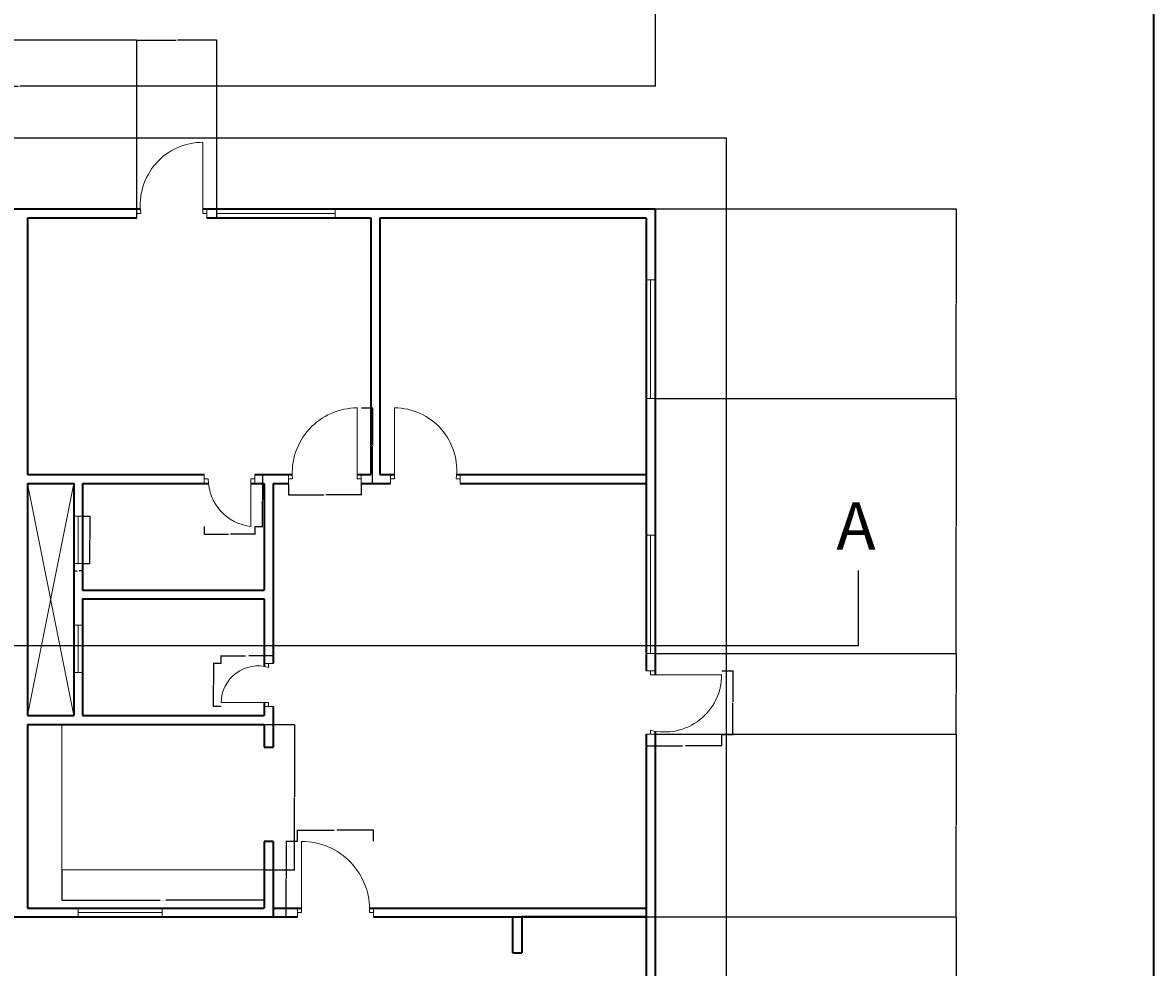
# Model space of a CAD drawing. Units: inches. Extents: x 1520 to 3401, y 1570 to 3432.
# Tile 14 of 15: x 2828 to 3401, y 2313 to 2791. Entities that reach past the tile are written whole.
import ezdxf

# ---------------------------------------------------------------- set-up
doc = ezdxf.new("R2010")
doc.units = ezdxf.units.IN
for name, color, linetype, lineweight in [('A-ANNO-DIMS', 2, 'Continuous', 18), ('A-ANNO-SYMB', 2, 'Continuous', 25), ('A-ANNO-TTLB', 7, 'Continuous', 35), ('A-DOOR', 3, 'Continuous', 18), ('A-FLOR-CASE', 8, 'Continuous', 18), ('A-FLOR-EDGE', 7, 'Continuous', 25), ('A-FLOR-EVTR', 7, 'Continuous', 35), ('A-FLOR-OPEN', 8, 'Continuous', 13), ('A-GLAZ', 4, 'Continuous', 18), ('A-WALL', 7, 'Continuous', 35)]:
    doc.layers.add(name, color=color, linetype=linetype, lineweight=lineweight)
doc.styles.get("Standard").update_dxf_attribs({"font": 'arial.ttf'})
doc.dimstyles.get("Standard").update_dxf_attribs({"dimtxt": 0.18, "dimasz": 0.18, "dimexe": 0.18, "dimexo": 0.0625, "dimgap": 0.09, "dimtad": 0, "dimtih": 1, "dimtoh": 1, "dimdec": 4, "dimzin": 0, "dimdsep": 46, "dimtxsty": 'Standard', "dimcen": 0.09, "dimadec": 0, "dimazin": 0, "dimtfac": 1, "dimtdec": 4, "dimtofl": 0, "dimtmove": 0, "dimatfit": 3, "dimfxl": 1, "dimtolj": 1, "dimtzin": 0, "dimarcsym": 0})

# ---------------------------------------------------------------- blocks, each defined once
blk = doc.blocks.new('DOOR-SWING-36-05')
for p, q in [((34.83, 2.25), (34.83, 38.25)), ((0, 4.5), (0, 4.5)), ((0, 4.5), (0, 0)), ((0, 0), (0, 2.25)), ((0, 2.25), (2, 2.25)), ((36.83, 2.25), (34.83, 2.25)), ((36.83, 4.5), (36.83, 0)), ((36.83, 0), (36.83, 2.25))]:
    blk.add_line(p, q)
blk.add_arc((34.83, 5.28), 32.97, 90, 185.2728)
blk = doc.blocks.new('DOOR-SWING-36-06')
for p, q in [((2, 2.25), (2, 38.25)), ((0, 4.5), (0, 0)), ((0, 0), (0, 2.25)), ((0, 2.25), (2, 2.25)), ((35.31, 2.25), (33.31, 2.25)), ((35.31, 4.5), (35.31, 0)), ((35.31, 0), (35.31, 2.25))]:
    blk.add_line(p, q)
blk.add_arc((2, 6.63), 31.62, 352.0372, 90)
blk = doc.blocks.new('DOOR-SWING-24-07')
for p, q in [((21.75, 21.72), (26.25, 21.72)), ((26.25, 21.72), (24, 21.72)), ((24, 21.72), (24, 19.72)), ((24, 2), (0, 2)), ((21.75, 0), (26.25, 0)), ((24, 0), (24, 2)), ((26.25, 0), (24, 0))]:
    blk.add_line(p, q)
blk.add_arc((18.54, 2), 18.54, 72.8832, 180)
blk = doc.blocks.new('DOOR-SWING-24-08')
for p, q in [((0, 26.25), (0, 21.75)), ((0, 21.75), (0, 24)), ((0, 24), (2, 24)), ((25.6, 24), (23.6, 24)), ((23.6, 24), (23.6, 0)), ((25.6, 21.75), (25.6, 26.25)), ((25.6, 26.25), (25.6, 24))]:
    blk.add_line(p, q)
blk.add_arc((26.13, 24), 24.13, 180, 263.9827)
blk = doc.blocks.new('DOOR-SWING-36-20')
for p, q in [((2, 2.25), (2, 38.25)), ((0, 4.5), (0, 0)), ((0, 0), (0, 2.25)), ((0, 2.25), (2, 2.25)), ((38.43, 2.25), (36.43, 2.25)), ((38.43, 4.5), (38.43, 0)), ((38.43, 0), (38.43, 2.25))]:
    blk.add_line(p, q)
blk.add_arc((2, 3.79), 34.46, 357.4431, 90)
blk = doc.blocks.new('DOOR-SWING-36-21')
for p, q in [((33.5, 2.25), (33.5, 38.25)), ((0, 4.5), (0, 0)), ((0, 0), (0, 2.25)), ((0, 2.25), (2, 2.25)), ((35.5, 2.25), (33.5, 2.25)), ((35.5, 0), (35.5, 4.5)), ((35.5, 4.5), (35.5, 2.25))]:
    blk.add_line(p, q)
blk.add_arc((33.5, 6.47), 31.78, 90, 187.6316)
blk = doc.blocks.new('DOOR-SWING-36-23')
for p, q in [((0, 32.12), (4.5, 32.12)), ((4.5, 32.12), (2.25, 32.12)), ((2.25, 32.12), (2.25, 30.12)), ((2.25, 30.12), (38.25, 30.12)), ((4.5, 0), (0, 0)), ((0, 0), (2.25, 0)), ((2.25, 0), (2.25, 2))]:
    blk.add_line(p, q)
blk.add_arc((9.27, 30.12), 28.98, 255.986, 0)
blk = doc.blocks.new('WIN-PLAN-24-01')
for p, q in [((0, 4.5), (0, 0)), ((0, 0), (0, 2.25)), ((0, 2.25), (24, 2.25)), ((24, 2.25), (24, 4.5)), ((24, 4.5), (24, 0))]:
    blk.add_line(p, q)
blk = doc.blocks.new('WIN-PLAN-60-02')
for p, q in [((4.5, 60), (0, 60)), ((0, 60), (2.25, 60)), ((2.25, 60), (2.25, 0)), ((4.5, 0), (0, 0)), ((2.25, 0), (4.5, 0))]:
    blk.add_line(p, q)
blk = doc.blocks.new('WIN-PLAN-60-03')
for p, q in [((0, 2.25), (0, 4.5)), ((0, 4.5), (0, 0)), ((60, 2.25), (0, 2.25)), ((60, 0), (60, 4.5)), ((60, 4.5), (60, 2.25))]:
    blk.add_line(p, q)
blk = doc.blocks.new('WIN-PLAN-24-07')
for p, q in [((2.25, 24), (0, 24)), ((0, 24), (4.5, 24)), ((2.25, 0), (2.25, 24)), ((4.5, 0), (0, 0)), ((0, 0), (4.5, 0)), ((4.5, 0), (2.25, 0))]:
    blk.add_line(p, q)
blk = doc.blocks.new('WIN-PLAN-42.5-08')
for p, q in [((0, 4.5), (0, 0)), ((0, 0), (0, 2.25)), ((0, 2.25), (0, 2.25)), ((0, 2.25), (42.53, 2.25)), ((42.53, 0), (42.53, 4.5))]:
    blk.add_line(p, q)
blk = doc.blocks.new('KITCHEN-COUNTER-03')
for p, q in [((0, 0), (0, 73.56)), ((102.45, 0), (0, 0))]:
    blk.add_line(p, q)
blk = doc.blocks.new('*D89')
at = {"layer": 'A-ANNO-DIMS', "color": 0, "lineweight": -2, "transparency": 16777216}
for p, q in [((2999.61, 2596.43), (3005.47, 2596.43)), ((3005.29, 2596.25), (3005.29, 2577.49)), ((3005.29, 2558.36), (3005.29, 2577.12)), ((2999.61, 2558.18), (3005.47, 2558.18))]:
    blk.add_line(p, q, dxfattribs=at)
at = {"layer": 'A-ANNO-DIMS', "color": 0, "transparency": 16777216}
for points in [[(3005.26, 2596.25), (3005.32, 2596.25), (3005.29, 2596.43)], [(3005.26, 2558.36), (3005.32, 2558.36), (3005.29, 2558.18)]]:
    blk.add_solid(points, dxfattribs=at)
at = {"layer": 'Defpoints', "color": 0, "transparency": 16777216}
for p in [(2999.55, 2596.43), (3005.29, 2596.43), (2999.55, 2558.18)]:
    blk.add_point(p, dxfattribs=at)
at = {"layer": 'A-ANNO-DIMS', "color": 0, "transparency": 16777216, "insert": (3005.29, 2577.3), "char_height": 0.18, "attachment_point": 5}
blk.add_mtext('\\A1;D05 38 TYP.', dxfattribs=at)
blk = doc.blocks.new('*D90')
at = {"layer": 'A-ANNO-DIMS', "color": 0, "lineweight": -2, "transparency": 16777216}
for p, q in [((2962.72, 2558.12), (2962.72, 2552.26)), ((2999.55, 2558.12), (2999.55, 2552.26)), ((2962.9, 2552.44), (2980.61, 2552.44)), ((2999.37, 2552.44), (2981.66, 2552.44))]:
    blk.add_line(p, q, dxfattribs=at)
at = {"layer": 'A-ANNO-DIMS', "color": 0, "transparency": 16777216}
for points in [[(2962.9, 2552.47), (2962.9, 2552.41), (2962.72, 2552.44)], [(2999.37, 2552.47), (2999.37, 2552.41), (2999.55, 2552.44)]]:
    blk.add_solid(points, dxfattribs=at)
at = {"layer": 'Defpoints', "color": 0, "transparency": 16777216}
for p in [(2962.72, 2558.18), (2999.55, 2558.18), (2999.55, 2552.44)]:
    blk.add_point(p, dxfattribs=at)
at = {"layer": 'A-ANNO-DIMS', "color": 0, "transparency": 16777216, "insert": (2981.14, 2552.44), "char_height": 0.18, "attachment_point": 5}
blk.add_mtext('\\A1;37 TYP.', dxfattribs=at)
blk = doc.blocks.new('*D93')
at = {"layer": 'A-ANNO-DIMS', "color": 0, "lineweight": -2, "transparency": 16777216}
for p, q in [((2928.65, 2467.04), (2928.65, 2471.1)), ((2928.83, 2470.92), (2940.98, 2470.92)), ((2954.72, 2470.92), (2942.56, 2470.92)), ((2954.9, 2467.04), (2954.9, 2471.1))]:
    blk.add_line(p, q, dxfattribs=at)
at = {"layer": 'A-ANNO-DIMS', "color": 0, "transparency": 16777216}
for points in [[(2928.83, 2470.95), (2928.83, 2470.89), (2928.65, 2470.92)], [(2954.72, 2470.95), (2954.72, 2470.89), (2954.9, 2470.92)]]:
    blk.add_solid(points, dxfattribs=at)
at = {"layer": 'Defpoints', "color": 0, "transparency": 16777216}
for p in [(2954.9, 2470.92), (2928.65, 2466.98), (2954.9, 2466.98)]:
    blk.add_point(p, dxfattribs=at)
at = {"layer": 'A-ANNO-DIMS', "color": 0, "transparency": 16777216, "insert": (2941.77, 2470.92), "char_height": 0.18, "attachment_point": 5}
blk.add_mtext('\\A1;D07 26 TYP.', dxfattribs=at)
blk = doc.blocks.new('*D94')
at = {"layer": 'A-ANNO-DIMS', "color": 0, "lineweight": -2, "transparency": 16777216}
for p, q in [((2928.59, 2466.98), (2924.53, 2466.98)), ((2924.71, 2466.8), (2924.71, 2456.3)), ((2924.71, 2445.44), (2924.71, 2455.94)), ((2928.59, 2445.26), (2924.53, 2445.26))]:
    blk.add_line(p, q, dxfattribs=at)
at = {"layer": 'A-ANNO-DIMS', "color": 0, "transparency": 16777216}
for points in [[(2924.68, 2466.8), (2924.74, 2466.8), (2924.71, 2466.98)], [(2924.68, 2445.44), (2924.74, 2445.44), (2924.71, 2445.26)]]:
    blk.add_solid(points, dxfattribs=at)
at = {"layer": 'Defpoints', "color": 0, "transparency": 16777216}
for p in [(2924.71, 2466.98), (2928.65, 2466.98), (2928.65, 2445.26)]:
    blk.add_point(p, dxfattribs=at)
at = {"layer": 'A-ANNO-DIMS', "color": 0, "transparency": 16777216, "insert": (2924.71, 2456.12), "char_height": 0.18, "attachment_point": 5}
blk.add_mtext('\\A1;22 TYP.', dxfattribs=at)
blk = doc.blocks.new('*D95')
at = {"layer": 'A-ANNO-DIMS', "color": 0, "lineweight": -2, "transparency": 16777216}
for p, q in [((2945.71, 2562.68), (2949.77, 2562.68)), ((2949.59, 2562.5), (2949.59, 2549.74)), ((2949.59, 2536.61), (2949.59, 2549.37)), ((2945.71, 2536.43), (2949.77, 2536.43))]:
    blk.add_line(p, q, dxfattribs=at)
at = {"layer": 'A-ANNO-DIMS', "color": 0, "transparency": 16777216}
for points in [[(2949.56, 2562.5), (2949.62, 2562.5), (2949.59, 2562.68)], [(2949.56, 2536.61), (2949.62, 2536.61), (2949.59, 2536.43)]]:
    blk.add_solid(points, dxfattribs=at)
at = {"layer": 'Defpoints', "color": 0, "transparency": 16777216}
for p in [(2945.65, 2562.68), (2949.59, 2562.68), (2945.65, 2536.43)]:
    blk.add_point(p, dxfattribs=at)
at = {"layer": 'A-ANNO-DIMS', "color": 0, "transparency": 16777216, "insert": (2949.59, 2549.55), "char_height": 0.18, "attachment_point": 5}
blk.add_mtext('\\A1;D08 26 TYP.', dxfattribs=at)
blk = doc.blocks.new('*D96')
at = {"layer": 'A-ANNO-DIMS', "color": 0, "lineweight": -2, "transparency": 16777216}
for p, q in [((2920.05, 2536.37), (2920.05, 2532.31)), ((2920.23, 2532.49), (2932.32, 2532.49)), ((2945.47, 2532.49), (2933.38, 2532.49)), ((2945.65, 2536.37), (2945.65, 2532.31))]:
    blk.add_line(p, q, dxfattribs=at)
at = {"layer": 'A-ANNO-DIMS', "color": 0, "transparency": 16777216}
for points in [[(2920.23, 2532.52), (2920.23, 2532.46), (2920.05, 2532.49)], [(2945.47, 2532.52), (2945.47, 2532.46), (2945.65, 2532.49)]]:
    blk.add_solid(points, dxfattribs=at)
at = {"layer": 'Defpoints', "color": 0, "transparency": 16777216}
for p in [(2920.05, 2536.43), (2945.65, 2536.43), (2945.65, 2532.49)]:
    blk.add_point(p, dxfattribs=at)
at = {"layer": 'A-ANNO-DIMS', "color": 0, "transparency": 16777216, "insert": (2932.85, 2532.49), "char_height": 0.18, "attachment_point": 5}
blk.add_mtext('\\A1;26 TYP.', dxfattribs=at)
blk = doc.blocks.new('*D119')
at = {"layer": 'A-ANNO-DIMS', "color": 0, "lineweight": -2, "transparency": 16777216}
for p, q in [((2967.34, 2376.99), (2967.34, 2382.87)), ((2967.52, 2382.69), (2985.76, 2382.69)), ((3005.59, 2382.69), (2987.34, 2382.69)), ((3005.77, 2376.99), (3005.77, 2382.87))]:
    blk.add_line(p, q, dxfattribs=at)
at = {"layer": 'A-ANNO-DIMS', "color": 0, "transparency": 16777216}
for points in [[(2967.52, 2382.72), (2967.52, 2382.66), (2967.34, 2382.69)], [(3005.59, 2382.72), (3005.59, 2382.66), (3005.77, 2382.69)]]:
    blk.add_solid(points, dxfattribs=at)
at = {"layer": 'Defpoints', "color": 0, "transparency": 16777216}
for p in [(3005.77, 2382.69), (2967.34, 2376.93), (3005.77, 2376.93)]:
    blk.add_point(p, dxfattribs=at)
at = {"layer": 'A-ANNO-DIMS', "color": 0, "transparency": 16777216, "insert": (2986.55, 2382.69), "char_height": 0.18, "attachment_point": 5}
blk.add_mtext('\\A1;D20 38 TYP.', dxfattribs=at)
blk = doc.blocks.new('*D120')
at = {"layer": 'A-ANNO-DIMS', "color": 0, "lineweight": -2, "transparency": 16777216}
for p, q in [((2967.28, 2376.93), (2961.39, 2376.93)), ((2961.57, 2376.75), (2961.57, 2357.99)), ((2961.57, 2338.86), (2961.57, 2357.62)), ((2967.28, 2338.68), (2961.39, 2338.68))]:
    blk.add_line(p, q, dxfattribs=at)
at = {"layer": 'A-ANNO-DIMS', "color": 0, "transparency": 16777216}
for points in [[(2961.54, 2376.75), (2961.6, 2376.75), (2961.57, 2376.93)], [(2961.54, 2338.86), (2961.6, 2338.86), (2961.57, 2338.68)]]:
    blk.add_solid(points, dxfattribs=at)
at = {"layer": 'Defpoints', "color": 0, "transparency": 16777216}
for p in [(2961.57, 2376.93), (2967.34, 2376.93), (2967.34, 2338.68)]:
    blk.add_point(p, dxfattribs=at)
at = {"layer": 'A-ANNO-DIMS', "color": 0, "transparency": 16777216, "insert": (2961.57, 2357.8), "char_height": 0.18, "attachment_point": 5}
blk.add_mtext('\\A1;38 TYP.', dxfattribs=at)
blk = doc.blocks.new('*D125')
at = {"layer": 'A-ANNO-DIMS', "color": 0, "lineweight": -2, "transparency": 16777216}
for p, q in [((3143.9, 2430.96), (3143.9, 2425.11)), ((3182.15, 2430.96), (3182.15, 2425.11)), ((3144.08, 2425.29), (3162.23, 2425.29)), ((3181.97, 2425.29), (3163.81, 2425.29))]:
    blk.add_line(p, q, dxfattribs=at)
at = {"layer": 'A-ANNO-DIMS', "color": 0, "transparency": 16777216}
for points in [[(3144.08, 2425.32), (3144.08, 2425.26), (3143.9, 2425.29)], [(3181.97, 2425.32), (3181.97, 2425.26), (3182.15, 2425.29)]]:
    blk.add_solid(points, dxfattribs=at)
at = {"layer": 'Defpoints', "color": 0, "transparency": 16777216}
for p in [(3143.9, 2431.03), (3182.15, 2431.03), (3182.15, 2425.29)]:
    blk.add_point(p, dxfattribs=at)
at = {"layer": 'A-ANNO-DIMS', "color": 0, "transparency": 16777216, "insert": (3163.02, 2425.29), "char_height": 0.18, "attachment_point": 5}
blk.add_mtext('\\A1;D23 38 TYP.', dxfattribs=at)
blk = doc.blocks.new('*D126')
at = {"layer": 'A-ANNO-DIMS', "color": 0, "lineweight": -2, "transparency": 16777216}
for p, q in [((3182.21, 2463.31), (3188.07, 2463.31)), ((3187.89, 2463.13), (3187.89, 2447.35)), ((3187.89, 2431.21), (3187.89, 2446.98)), ((3182.21, 2431.03), (3188.07, 2431.03))]:
    blk.add_line(p, q, dxfattribs=at)
at = {"layer": 'A-ANNO-DIMS', "color": 0, "transparency": 16777216}
for points in [[(3187.86, 2463.13), (3187.92, 2463.13), (3187.89, 2463.31)], [(3187.86, 2431.21), (3187.92, 2431.21), (3187.89, 2431.03)]]:
    blk.add_solid(points, dxfattribs=at)
at = {"layer": 'Defpoints', "color": 0, "transparency": 16777216}
for p in [(3182.15, 2463.31), (3187.89, 2463.31), (3182.15, 2431.03)]:
    blk.add_point(p, dxfattribs=at)
at = {"layer": 'A-ANNO-DIMS', "color": 0, "transparency": 16777216, "insert": (3187.89, 2447.17), "char_height": 0.18, "attachment_point": 5}
blk.add_mtext('\\A1;32 TYP.', dxfattribs=at)
blk = doc.blocks.new('*D145')
at = {"layer": 'A-ANNO-DIMS', "color": 0, "lineweight": -2, "transparency": 16777216}
for p, q in [((2858.46, 2541.57), (2862.18, 2541.57)), ((2862, 2541.39), (2862, 2529.75)), ((2862, 2517.75), (2862, 2529.39)), ((2858.46, 2517.57), (2862.18, 2517.57))]:
    blk.add_line(p, q, dxfattribs=at)
at = {"layer": 'A-ANNO-DIMS', "color": 0, "transparency": 16777216}
for points in [[(2861.97, 2541.39), (2862.03, 2541.39), (2862, 2541.57)], [(2861.97, 2517.75), (2862.03, 2517.75), (2862, 2517.57)]]:
    blk.add_solid(points, dxfattribs=at)
at = {"layer": 'Defpoints', "color": 0, "transparency": 16777216}
for p in [(2858.4, 2541.57), (2862, 2541.57), (2858.4, 2517.57)]:
    blk.add_point(p, dxfattribs=at)
at = {"layer": 'A-ANNO-DIMS', "color": 0, "transparency": 16777216, "insert": (2862, 2529.57), "char_height": 0.18, "attachment_point": 5}
blk.add_mtext('\\A1;W7 24 TYP.', dxfattribs=at)
blk = doc.blocks.new('*D146')
at = {"layer": 'A-ANNO-DIMS', "color": 0, "lineweight": -2, "transparency": 16777216}
for p, q in [((2853.9, 2517.5), (2853.9, 2513.79)), ((2858.4, 2517.5), (2858.4, 2513.79)), ((2854.08, 2513.97), (2855.69, 2513.97)), ((2858.22, 2513.97), (2856.61, 2513.97))]:
    blk.add_line(p, q, dxfattribs=at)
at = {"layer": 'A-ANNO-DIMS', "color": 0, "transparency": 16777216}
for points in [[(2854.08, 2514), (2854.08, 2513.94), (2853.9, 2513.97)], [(2858.22, 2514), (2858.22, 2513.94), (2858.4, 2513.97)]]:
    blk.add_solid(points, dxfattribs=at)
at = {"layer": 'Defpoints', "color": 0, "transparency": 16777216}
for p in [(2853.9, 2517.57), (2858.4, 2517.57), (2858.4, 2513.97)]:
    blk.add_point(p, dxfattribs=at)
at = {"layer": 'A-ANNO-DIMS', "color": 0, "transparency": 16777216, "insert": (2856.15, 2513.97), "char_height": 0.18, "attachment_point": 5}
blk.add_mtext('\\A1;5 TYP.', dxfattribs=at)
blk = doc.blocks.new('*D153')
at = {"layer": 'A-ANNO-DIMS', "color": 0, "lineweight": -2, "transparency": 16777216}
for p, q in [((2847.95, 2362.55), (2847.95, 2347.07)), ((2950.4, 2362.55), (2950.4, 2347.07)), ((2848.13, 2347.25), (2897.72, 2347.25)), ((2950.22, 2347.25), (2900.62, 2347.25))]:
    blk.add_line(p, q, dxfattribs=at)
at = {"layer": 'A-ANNO-DIMS', "color": 0, "transparency": 16777216}
for points in [[(2848.13, 2347.28), (2848.13, 2347.22), (2847.95, 2347.25)], [(2950.22, 2347.28), (2950.22, 2347.22), (2950.4, 2347.25)]]:
    blk.add_solid(points, dxfattribs=at)
at = {"layer": 'Defpoints', "color": 0, "transparency": 16777216}
for p in [(2847.95, 2362.61), (2950.4, 2362.61), (2950.4, 2347.25)]:
    blk.add_point(p, dxfattribs=at)
at = {"layer": 'A-ANNO-DIMS', "color": 0, "transparency": 16777216, "insert": (2899.17, 2347.25), "char_height": 0.18, "attachment_point": 5}
blk.add_mtext('\\A1;COUNTER C3 102 TYP.', dxfattribs=at)
blk = doc.blocks.new('*D154')
at = {"layer": 'A-ANNO-DIMS', "color": 0, "lineweight": -2, "transparency": 16777216}
for p, q in [((2950.46, 2436.18), (2965.95, 2436.18)), ((2965.77, 2436), (2965.77, 2399.58)), ((2965.77, 2362.79), (2965.77, 2399.22)), ((2950.46, 2362.61), (2965.95, 2362.61))]:
    blk.add_line(p, q, dxfattribs=at)
at = {"layer": 'A-ANNO-DIMS', "color": 0, "transparency": 16777216}
for points in [[(2965.74, 2436), (2965.8, 2436), (2965.77, 2436.18)], [(2965.74, 2362.79), (2965.8, 2362.79), (2965.77, 2362.61)]]:
    blk.add_solid(points, dxfattribs=at)
at = {"layer": 'Defpoints', "color": 0, "transparency": 16777216}
for p in [(2950.4, 2436.18), (2965.77, 2436.18), (2950.4, 2362.61)]:
    blk.add_point(p, dxfattribs=at)
at = {"layer": 'A-ANNO-DIMS', "color": 0, "transparency": 16777216, "insert": (2965.77, 2399.4), "char_height": 0.18, "attachment_point": 5}
blk.add_mtext('\\A1;74 TYP.', dxfattribs=at)
blk = doc.blocks.new('*D197')
at = {"layer": 'A-ANNO-DIMS', "color": 0, "lineweight": -2, "transparency": 16777216}
for p, q in [((3143.96, 2338.68), (3301.09, 2338.68)), ((3300.91, 2338.5), (3300.91, 2288.86)), ((3300.91, 2238.86), (3300.91, 2288.5)), ((3143.96, 2238.68), (3301.09, 2238.68))]:
    blk.add_line(p, q, dxfattribs=at)
at = {"layer": 'A-ANNO-DIMS', "color": 0, "transparency": 16777216}
for points in [[(3300.88, 2338.5), (3300.94, 2338.5), (3300.91, 2338.68)], [(3300.88, 2238.86), (3300.94, 2238.86), (3300.91, 2238.68)]]:
    blk.add_solid(points, dxfattribs=at)
at = {"layer": 'Defpoints', "color": 0, "transparency": 16777216}
for p in [(3143.9, 2338.68), (3300.91, 2338.68), (3143.9, 2238.68)]:
    blk.add_point(p, dxfattribs=at)
at = {"layer": 'A-ANNO-DIMS', "color": 0, "transparency": 16777216, "insert": (3300.91, 2288.68), "char_height": 0.18, "attachment_point": 5}
blk.add_mtext('\\A1;100', dxfattribs=at)
blk = doc.blocks.new('*D198')
at = {"layer": 'A-ANNO-DIMS', "color": 0, "lineweight": -2, "transparency": 16777216}
for p, q in [((3148.46, 2431.19), (3301.09, 2431.19)), ((3300.91, 2431.01), (3300.91, 2385.11)), ((3300.91, 2338.86), (3300.91, 2384.75)), ((3143.96, 2338.68), (3301.09, 2338.68))]:
    blk.add_line(p, q, dxfattribs=at)
at = {"layer": 'A-ANNO-DIMS', "color": 0, "transparency": 16777216}
for points in [[(3300.88, 2431.01), (3300.94, 2431.01), (3300.91, 2431.19)], [(3300.88, 2338.86), (3300.94, 2338.86), (3300.91, 2338.68)]]:
    blk.add_solid(points, dxfattribs=at)
at = {"layer": 'Defpoints', "color": 0, "transparency": 16777216}
for p in [(3148.4, 2431.19), (3300.91, 2431.19), (3143.9, 2338.68)]:
    blk.add_point(p, dxfattribs=at)
at = {"layer": 'A-ANNO-DIMS', "color": 0, "transparency": 16777216, "insert": (3300.91, 2384.93), "char_height": 0.18, "attachment_point": 5}
blk.add_mtext('\\A1;92.5', dxfattribs=at)
blk = doc.blocks.new('*D199')
at = {"layer": 'A-ANNO-DIMS', "color": 0, "lineweight": -2, "transparency": 16777216}
for p, q in [((3148.46, 2472.01), (3301.09, 2472.01)), ((3300.91, 2471.83), (3300.91, 2451.78)), ((3300.91, 2431.37), (3300.91, 2451.42)), ((3148.46, 2431.19), (3301.09, 2431.19))]:
    blk.add_line(p, q, dxfattribs=at)
at = {"layer": 'A-ANNO-DIMS', "color": 0, "transparency": 16777216}
for points in [[(3300.88, 2471.83), (3300.94, 2471.83), (3300.91, 2472.01)], [(3300.88, 2431.37), (3300.94, 2431.37), (3300.91, 2431.19)]]:
    blk.add_solid(points, dxfattribs=at)
at = {"layer": 'Defpoints', "color": 0, "transparency": 16777216}
for p in [(3148.4, 2472.01), (3300.91, 2472.01), (3148.4, 2431.19)]:
    blk.add_point(p, dxfattribs=at)
at = {"layer": 'A-ANNO-DIMS', "color": 0, "transparency": 16777216, "insert": (3300.91, 2451.6), "char_height": 0.18, "attachment_point": 5}
blk.add_mtext('\\A1;40.83', dxfattribs=at)
blk = doc.blocks.new('*D200')
at = {"layer": 'A-ANNO-DIMS', "color": 0, "lineweight": -2, "transparency": 16777216}
for p, q in [((3148.46, 2601.18), (3301.09, 2601.18)), ((3300.91, 2601), (3300.91, 2536.78)), ((3300.91, 2472.19), (3300.91, 2536.42)), ((3148.46, 2472.01), (3301.09, 2472.01))]:
    blk.add_line(p, q, dxfattribs=at)
at = {"layer": 'A-ANNO-DIMS', "color": 0, "transparency": 16777216}
for points in [[(3300.88, 2601), (3300.94, 2601), (3300.91, 2601.18)], [(3300.88, 2472.19), (3300.94, 2472.19), (3300.91, 2472.01)]]:
    blk.add_solid(points, dxfattribs=at)
at = {"layer": 'Defpoints', "color": 0, "transparency": 16777216}
for p in [(3148.4, 2601.18), (3300.91, 2601.18), (3148.4, 2472.01)]:
    blk.add_point(p, dxfattribs=at)
at = {"layer": 'A-ANNO-DIMS', "color": 0, "transparency": 16777216, "insert": (3300.91, 2536.6), "char_height": 0.18, "attachment_point": 5}
blk.add_mtext('\\A1;129.17', dxfattribs=at)
blk = doc.blocks.new('*D201')
at = {"layer": 'A-ANNO-DIMS', "color": 0, "lineweight": -2, "transparency": 16777216}
for p, q in [((3148.46, 2697.18), (3301.09, 2697.18)), ((3300.91, 2697), (3300.91, 2649.36)), ((3300.91, 2601.36), (3300.91, 2649)), ((3148.46, 2601.18), (3301.09, 2601.18))]:
    blk.add_line(p, q, dxfattribs=at)
at = {"layer": 'A-ANNO-DIMS', "color": 0, "transparency": 16777216}
for points in [[(3300.88, 2697), (3300.94, 2697), (3300.91, 2697.18)], [(3300.88, 2601.36), (3300.94, 2601.36), (3300.91, 2601.18)]]:
    blk.add_solid(points, dxfattribs=at)
at = {"layer": 'Defpoints', "color": 0, "transparency": 16777216}
for p in [(3148.4, 2697.18), (3300.91, 2697.18), (3148.4, 2601.18)]:
    blk.add_point(p, dxfattribs=at)
at = {"layer": 'A-ANNO-DIMS', "color": 0, "transparency": 16777216, "insert": (3300.91, 2649.18), "char_height": 0.18, "attachment_point": 5}
blk.add_mtext('\\A1;96', dxfattribs=at)
blk = doc.blocks.new('*D205')
at = {"layer": 'A-ANNO-DIMS', "color": 0, "lineweight": -2, "transparency": 16777216}
for p, q in [((2733.5, 2697.24), (2733.5, 2782.76)), ((2733.68, 2782.58), (2809.22, 2782.58)), ((2885.68, 2782.58), (2810.13, 2782.58)), ((2885.86, 2692.74), (2885.86, 2782.76))]:
    blk.add_line(p, q, dxfattribs=at)
at = {"layer": 'A-ANNO-DIMS', "color": 0, "transparency": 16777216}
for points in [[(2733.68, 2782.61), (2733.68, 2782.55), (2733.5, 2782.58)], [(2885.68, 2782.61), (2885.68, 2782.55), (2885.86, 2782.58)]]:
    blk.add_solid(points, dxfattribs=at)
at = {"layer": 'Defpoints', "color": 0, "transparency": 16777216}
for p in [(2885.86, 2782.58), (2733.5, 2697.18), (2885.86, 2692.68)]:
    blk.add_point(p, dxfattribs=at)
at = {"layer": 'A-ANNO-DIMS', "color": 0, "transparency": 16777216, "insert": (2809.68, 2782.58), "char_height": 0.18, "attachment_point": 5}
blk.add_mtext('\\A1;152.37', dxfattribs=at)
blk = doc.blocks.new('*D206')
at = {"layer": 'A-ANNO-DIMS', "color": 0, "lineweight": -2, "transparency": 16777216}
for p, q in [((2885.86, 2692.74), (2885.86, 2782.76)), ((2886.04, 2782.58), (2905.74, 2782.58)), ((2926.19, 2782.58), (2906.5, 2782.58)), ((2926.37, 2692.74), (2926.37, 2782.76))]:
    blk.add_line(p, q, dxfattribs=at)
at = {"layer": 'A-ANNO-DIMS', "color": 0, "transparency": 16777216}
for points in [[(2886.04, 2782.61), (2886.04, 2782.55), (2885.86, 2782.58)], [(2926.19, 2782.61), (2926.19, 2782.55), (2926.37, 2782.58)]]:
    blk.add_solid(points, dxfattribs=at)
at = {"layer": 'Defpoints', "color": 0, "transparency": 16777216}
for p in [(2926.37, 2782.58), (2885.86, 2692.68), (2926.37, 2692.68)]:
    blk.add_point(p, dxfattribs=at)
at = {"layer": 'A-ANNO-DIMS', "color": 0, "transparency": 16777216, "insert": (2906.12, 2782.58), "char_height": 0.18, "attachment_point": 5}
blk.add_mtext('\\A1;40.51', dxfattribs=at)
blk = doc.blocks.new('*D224')
at = {"layer": 'A-ANNO-DIMS', "color": 0, "lineweight": -2, "transparency": 16777216}
for p, q in [((2503.9, 2875.57), (2503.9, 2759.2)), ((3148.4, 2875.57), (3148.4, 2759.2)), ((2504.08, 2759.38), (2825.75, 2759.38)), ((3148.22, 2759.38), (2826.54, 2759.38))]:
    blk.add_line(p, q, dxfattribs=at)
at = {"layer": 'A-ANNO-DIMS', "color": 0, "transparency": 16777216}
for points in [[(2504.08, 2759.41), (2504.08, 2759.35), (2503.9, 2759.38)], [(3148.22, 2759.41), (3148.22, 2759.35), (3148.4, 2759.38)]]:
    blk.add_solid(points, dxfattribs=at)
at = {"layer": 'Defpoints', "color": 0, "transparency": 16777216}
for p in [(2503.9, 2875.63), (3148.4, 2875.63), (3148.4, 2759.38)]:
    blk.add_point(p, dxfattribs=at)
at = {"layer": 'A-ANNO-DIMS', "color": 0, "transparency": 16777216, "insert": (2826.15, 2759.38), "char_height": 0.18, "attachment_point": 5}
blk.add_mtext('\\A1;644.5', dxfattribs=at)

msp = doc.modelspace()

# ---------------------------------------------------------------- linework, layer by layer
at = {"layer": 'A-ANNO-SYMB'}
for p, q in [((3251.5148, 2476.123), (3251.5148, 2514.1695)), ((2435.8982, 2476.123), (3251.5148, 2476.123))]:
    msp.add_line(p, q, dxfattribs=at)
at = {"layer": 'A-ANNO-TTLB'}
msp.add_lwpolyline([(1519.9253, 3431.7421), (3400.8761, 3431.7421), (3400.8761, 1570.3458), (1519.9253, 1570.3458)], close=True, dxfattribs=at)
at = {"layer": 'A-FLOR-EDGE'}
for p, q in [((2467.8987, 2733.1786), (3184.3987, 2733.1786)), ((3184.3987, 2733.1786), (3184.3987, 1791.6786))]:
    msp.add_line(p, q, dxfattribs=at)
at = {"layer": 'A-FLOR-EVTR'}
for p, q in [((3076.3987, 2320.4639), (3076.3987, 2338.6786)), ((3143.8987, 2338.6786), (3080.8987, 2338.6786)), ((3080.8987, 2338.6786), (3080.8987, 2320.4639)), ((3076.3987, 2320.4639), (3080.8987, 2320.4639))]:
    msp.add_line(p, q, dxfattribs=at)
at = {"layer": 'A-FLOR-OPEN'}
for p, q in [((2853.8987, 2558.1786), (2830.3987, 2440.6786)), ((2830.3987, 2558.1786), (2853.8987, 2440.6786))]:
    msp.add_line(p, q, dxfattribs=at)
at = {"layer": 'A-WALL'}
for p, q in [((2611.6928, 2697.1786), (2887.6429, 2697.1786)), ((2830.3987, 2692.6786), (2830.3987, 2562.6786)), ((2830.3987, 2692.6786), (2885.8633, 2692.6786)), ((2919.3613, 2697.1786), (3148.3987, 2697.1786)), ((2921.3613, 2692.6786), (3004.3987, 2692.6786)), ((3004.3987, 2692.6786), (3004.3987, 2562.6786)), ((3008.8987, 2692.6786), (3008.8987, 2562.6786)), ((3008.8987, 2692.6786), (3143.8987, 2692.6786)), ((3143.8987, 2692.6786), (3143.8987, 2463.3065)), ((3148.3987, 2697.1786), (3148.3987, 2461.3065)), ((2830.3987, 2562.6786), (2920.0454, 2562.6786)), ((2945.6486, 2562.6786), (2964.5904, 2562.6786)), ((2997.5513, 2562.6786), (3004.3987, 2562.6786)), ((3008.8987, 2562.6786), (3016.3386, 2562.6786)), ((3047.8865, 2562.6786), (3143.8987, 2562.6786)), ((2830.3987, 2558.1786), (2830.3987, 2440.6786)), ((2830.3987, 2558.1786), (2853.8987, 2558.1786)), ((2853.8987, 2558.1786), (2853.8987, 2440.6786)), ((2858.3987, 2558.1786), (2858.3987, 2504.1786)), ((2858.3987, 2558.1786), (2922.1505, 2558.1786)), ((2943.6486, 2558.1786), (2950.3987, 2558.1786)), ((2950.3987, 2558.1786), (2950.3987, 2504.1786)), ((2954.8987, 2558.1786), (2954.8987, 2466.9777)), ((2954.8987, 2558.1786), (2962.7207, 2558.1786)), ((2999.5513, 2558.1786), (3014.3386, 2558.1786)), ((3049.6534, 2558.1786), (3143.8987, 2558.1786)), ((2858.3987, 2504.1786), (2950.3987, 2504.1786)), ((2858.3987, 2499.6786), (2858.3987, 2440.6786)), ((2858.3987, 2499.6786), (2950.3987, 2499.6786)), ((2950.3987, 2499.6786), (2950.3987, 2465.5195)), ((2950.3987, 2447.2565), (2950.3987, 2440.6786)), ((2830.3987, 2440.6786), (2853.8987, 2440.6786)), ((2858.3987, 2440.6786), (2950.3987, 2440.6786)), ((2954.8987, 2445.2565), (2954.8987, 2424.6989)), ((2830.3987, 2436.1786), (2830.3987, 2343.1786)), ((2830.3987, 2436.1786), (2950.3987, 2436.1786)), ((2950.3987, 2436.1786), (2950.3987, 2424.6989)), ((3143.8987, 2431.1873), (3143.8987, 1963.6868)), ((3148.3987, 2432.7197), (3148.3987, 1965.1342)), ((2950.3987, 2424.6989), (2954.8987, 2424.6989)), ((2950.3987, 2376.8563), (2950.3987, 2343.1786)), ((2954.8987, 2376.8563), (2950.3987, 2376.8563)), ((2954.8987, 2376.8563), (2954.8987, 2338.6786)), ((2830.3987, 2343.1786), (2950.3987, 2343.1786)), ((2954.8987, 2343.1786), (2969.3389, 2343.1786)), ((3003.7941, 2343.1786), (3143.8987, 2343.1786)), ((2817.9986, 2338.6786), (2967.3389, 2338.6786)), ((3005.7672, 2338.6786), (3143.8987, 2338.6786))]:
    msp.add_line(p, q, dxfattribs=at)

# ---------------------------------------------------------------- block references
at = {"layer": 'A-DOOR'}
for name, p in [('DOOR-SWING-36-21', (2885.8628, 2692.679)), ('DOOR-SWING-36-05', (2962.7208, 2558.179)), ('DOOR-SWING-36-06', (3014.3388, 2558.179)), ('DOOR-SWING-24-08', (2920.0458, 2536.429)), ('DOOR-SWING-24-07', (2928.6488, 2445.256)), ('DOOR-SWING-36-23', (3143.8988, 2431.187)), ('DOOR-SWING-36-20', (2967.3388, 2338.679))]:
    msp.add_blockref(name, p, dxfattribs=at)
at = {"layer": 'A-FLOR-CASE'}
msp.add_blockref('KITCHEN-COUNTER-03', (2847.9458, 2362.615), dxfattribs=at)
at = {"layer": 'A-GLAZ'}
for name, p in [('WIN-PLAN-60-03', (2926.3718, 2692.679)), ('WIN-PLAN-24-07', (2853.8988, 2517.567)), ('WIN-PLAN-42.5-08', (2856.1388, 2338.679))]:
    msp.add_blockref(name, p, dxfattribs=at)
at = {"layer": 'A-GLAZ', "extrusion": (0, 0, -1), "zscale": -1}
for name, p, rotation in [('WIN-PLAN-60-02', (-3143.8988, 2661.184), 180), ('WIN-PLAN-60-03', (-3143.899, 2472.0145), 90)]:
    msp.add_blockref(name, p, dxfattribs=dict(at, rotation=rotation))
at = {"layer": 'A-GLAZ', "rotation": 270}
msp.add_blockref('WIN-PLAN-24-01', (2853.899, 2486.4027), dxfattribs=at)

# ---------------------------------------------------------------- texts
at = {"layer": 'A-ANNO-SYMB', "insert": (3240.2547, 2548.6961), "char_height": 24, "attachment_point": 1}
msp.add_mtext_dynamic_manual_height_columns('A', width=40.019877, gutter_width=12.5, heights=[0], dxfattribs=at)

# ---------------------------------------------------------------- dimensions: what is measured, and where the dimension line sits
at = {"layer": 'A-ANNO-DIMS'}
for base, p1, p2, override, picture, middle in [((3148.3987, 2759.3805), (2503.8987, 2875.633), (3148.3987, 2875.633), {"dimdec": 1, "dimlfac": 1, "dimrnd": 0, "dimzin": 0, "dimdsep": 46, "dimlunit": 2}, '*D224', (2826.1487, 2759.3805)), ((2885.8633, 2782.5786), (2733.4955, 2697.1786), (2885.8633, 2692.6786), {"dimdec": 2, "dimlfac": 1, "dimrnd": 0, "dimzin": 0, "dimdsep": 46, "dimlunit": 2}, '*D205', (2809.6794, 2782.5786)), ((2926.372, 2782.5786), (2885.8633, 2692.6786), (2926.372, 2692.6786), {"dimdec": 2, "dimlfac": 1, "dimrnd": 0, "dimzin": 0, "dimdsep": 46, "dimlunit": 2}, '*D206', (2906.1176, 2782.5786))]:
    dim = msp.add_linear_dim(base=base, p1=p1, p2=p2, dimstyle='Standard', override=override, dxfattribs=at)
    dim.commit()
    dim.dimension.update_dxf_attribs({"geometry": picture, "text_midpoint": middle})
for base, p1, p2, override, picture, middle in [((3300.9148, 2697.1786), (3148.3987, 2601.1845), (3148.3987, 2697.1786), {"dimdec": 0, "dimlfac": 1, "dimrnd": 0, "dimzin": 0, "dimdsep": 46, "dimlunit": 2}, '*D201', (3300.9148, 2649.1816)), ((3300.9148, 2601.1845), (3148.3987, 2472.0146), (3148.3987, 2601.1845), {"dimdec": 2, "dimlfac": 1, "dimrnd": 0, "dimzin": 0, "dimdsep": 46, "dimlunit": 2}, '*D200', (3300.9148, 2536.5996)), ((3300.9148, 2472.0146), (3148.3987, 2431.1873), (3148.3987, 2472.0146), {"dimdec": 2, "dimlfac": 1, "dimrnd": 0, "dimzin": 0, "dimdsep": 46, "dimlunit": 2}, '*D199', (3300.9148, 2451.601)), ((3300.9148, 2431.1873), (3143.8987, 2338.6786), (3148.3987, 2431.1873), {"dimdec": 1, "dimlfac": 1, "dimrnd": 0, "dimzin": 0, "dimdsep": 46, "dimlunit": 2}, '*D198', (3300.9148, 2384.933)), ((3300.9148, 2338.6786), (3143.8987, 2238.6786), (3143.8987, 2338.6786), {"dimdec": 0, "dimlfac": 1, "dimrnd": 0, "dimzin": 0, "dimdsep": 46, "dimlunit": 2}, '*D197', (3300.9148, 2288.6786))]:
    dim = msp.add_linear_dim(base=base, p1=p1, p2=p2, angle=90, dimstyle='Standard', override=override, dxfattribs=at)
    dim.commit()
    dim.dimension.update_dxf_attribs({"geometry": picture, "text_midpoint": middle})
for base, p1, p2, text, picture, middle in [((3005.2888, 2596.4286), (2999.5513, 2558.1786), (2999.5513, 2596.4286), 'D05 <> TYP.', '*D89', (3005.2888, 2577.3036)), ((2949.5861, 2562.6786), (2945.6486, 2536.4286), (2945.6486, 2562.6786), 'D08 <> TYP.', '*D95', (2949.5861, 2549.5536)), ((2861.9987, 2541.5671), (2858.3987, 2517.5671), (2858.3987, 2541.5671), 'W7 <> TYP.', '*D145', (2861.9987, 2529.5671)), ((2924.7112, 2466.9777), (2928.6487, 2445.2565), (2928.6487, 2466.9777), '<> TYP.', '*D94', (2924.7112, 2456.1171)), ((3187.8862, 2463.3065), (3182.1487, 2431.0267), (3182.1487, 2463.3065), '<> TYP.', '*D126', (3187.8862, 2447.1666)), ((2965.7666, 2436.1786), (2950.3987, 2362.615), (2950.3987, 2436.1786), '<> TYP.', '*D154', (2965.7666, 2399.3968)), ((2961.5746, 2376.9286), (2967.3389, 2338.6786), (2967.3389, 2376.9286), '<> TYP.', '*D120', (2961.5746, 2357.8036))]:
    dim = msp.add_linear_dim(base=base, p1=p1, p2=p2, angle=90, text=text, dimstyle='Standard', override={"dimdec": 0, "dimlfac": 1, "dimrnd": 0, "dimzin": 0, "dimdsep": 46, "dimlunit": 2}, dxfattribs=at)
    dim.commit()
    dim.dimension.update_dxf_attribs({"geometry": picture, "text_midpoint": middle})
for base, p1, p2, text, picture, middle in [((2999.5513, 2552.4411), (2962.7207, 2558.1786), (2999.5513, 2558.1786), '<> TYP.', '*D90', (2981.136, 2552.4411)), ((2945.6486, 2532.4911), (2920.0454, 2536.4286), (2945.6486, 2536.4286), '<> TYP.', '*D96', (2932.847, 2532.4911)), ((2858.3986527147, 2513.9671218481), (2853.8986527147, 2517.5671218481), (2858.3986527147, 2517.5671218481), '<> TYP.', '*D146', (2856.1486527147, 2513.9671218481)), ((2954.8987, 2470.9152), (2928.6487, 2466.9777), (2954.8987, 2466.9777), 'D07 <> TYP.', '*D93', (2941.7737, 2470.9152)), ((3182.1487, 2425.2892), (3143.8987, 2431.0267), (3182.1487, 2431.0267), 'D23 <> TYP.', '*D125', (3163.0237, 2425.2892)), ((3005.7672, 2382.6929), (2967.3389, 2376.9286), (3005.7672, 2376.9286), 'D20 <> TYP.', '*D119', (2986.553, 2382.6929)), ((2950.3987, 2347.247), (2847.9454, 2362.615), (2950.3987, 2362.615), 'COUNTER C3 <> TYP.', '*D153', (2899.172, 2347.247))]:
    dim = msp.add_linear_dim(base=base, p1=p1, p2=p2, text=text, dimstyle='Standard', override={"dimdec": 0, "dimlfac": 1, "dimrnd": 0, "dimzin": 0, "dimdsep": 46, "dimlunit": 2}, dxfattribs=at)
    dim.commit()
    dim.dimension.update_dxf_attribs({"geometry": picture, "text_midpoint": middle})

doc.saveas('drawing.dxf')
